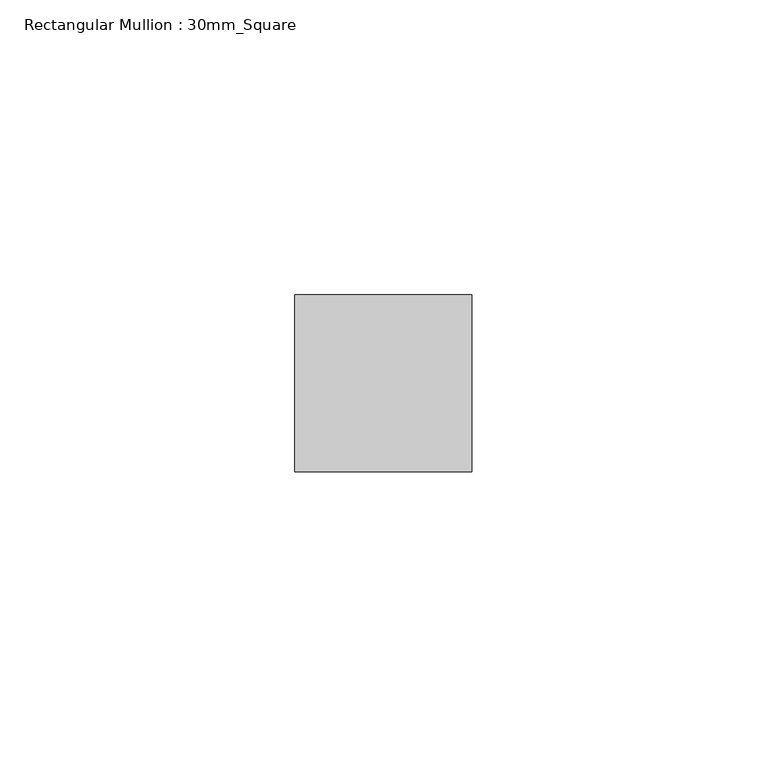
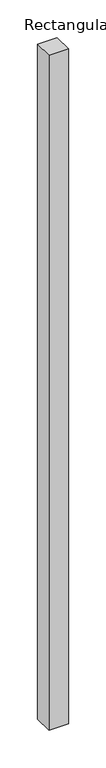
"""IFC4 building model written with IfcOpenShell, lengths in millimetres: member geometry, Rectangular Mullion : 30mm_Square."""

from ifc_helpers import new_model, si_unit, frame, origin, place, context, project, spatial, polyline, outline, extrude, source, transform, mapped, element, save


def rectangular_mullion_30mm_square_b25d63a0(model_context):
    return source(origin(), model_context, "Body", "SweptSolid", [
        extrude(outline(polyline([(15.0, 15.0), (15.0, -15.0), (-15.0, -15.0), (-15.0, 15.0), (15.0, 15.0)])), frame((0.0, 0.0, -1092.6063046), z_axis=(0.0, 0.0, 1.0), x_axis=(1.0, 0.0, 0.0)), (0.0, 0.0, 1.0), 1092.6063046),
    ])


if __name__ == "__main__":
    model = new_model("IFC4")
    model_context = context("Model", 3, world=origin())
    ifc_project = project(units=[si_unit("LENGTHUNIT", "METRE", prefix="MILLI")], contexts=[model_context])
    site = spatial("IfcSite", under=ifc_project)
    building = spatial("IfcBuilding", under=site)
    placement = place(None, origin())
    rectangular_mullion_30mm_square_shape = rectangular_mullion_30mm_square_b25d63a0(model_context)
    element("IfcMember", 1, ObjectType="Rectangular Mullion : 30mm_Square", at=placement, inside=building, context=model_context, shape_type="MappedRepresentation", body=[
        mapped(rectangular_mullion_30mm_square_shape, transform((0.0, 0.0, 0.0), x_axis=(1.0, 0.0, 0.0), y_axis=(0.0, 1.0, 0.0), z_axis=(0.0, 0.0, 1.0))),
    ])
    save(model, "model.ifc")

# Revit data of these elements
# Type "Rectangular Mullion : 30mm_Square"
#   Keynote = "H11"
#   built-in parameter 1007304 = 0.0984252 (stored number, unit not read)
#   built-in parameter 1007301 = 0.0492126 (stored number, unit not read)
#   built-in parameter 1007300 = 0.0492126 (stored number, unit not read)
# Element 1 (IfcMember, "Rectangular Mullion : 30mm_Square")
#   Materials on its faces: "Aluminium"
# Materials
#   "Aluminium": class "Metal", colour RGB 247 247 247, transparency 0, Description = "Aluminium 6061", Cost = 0
